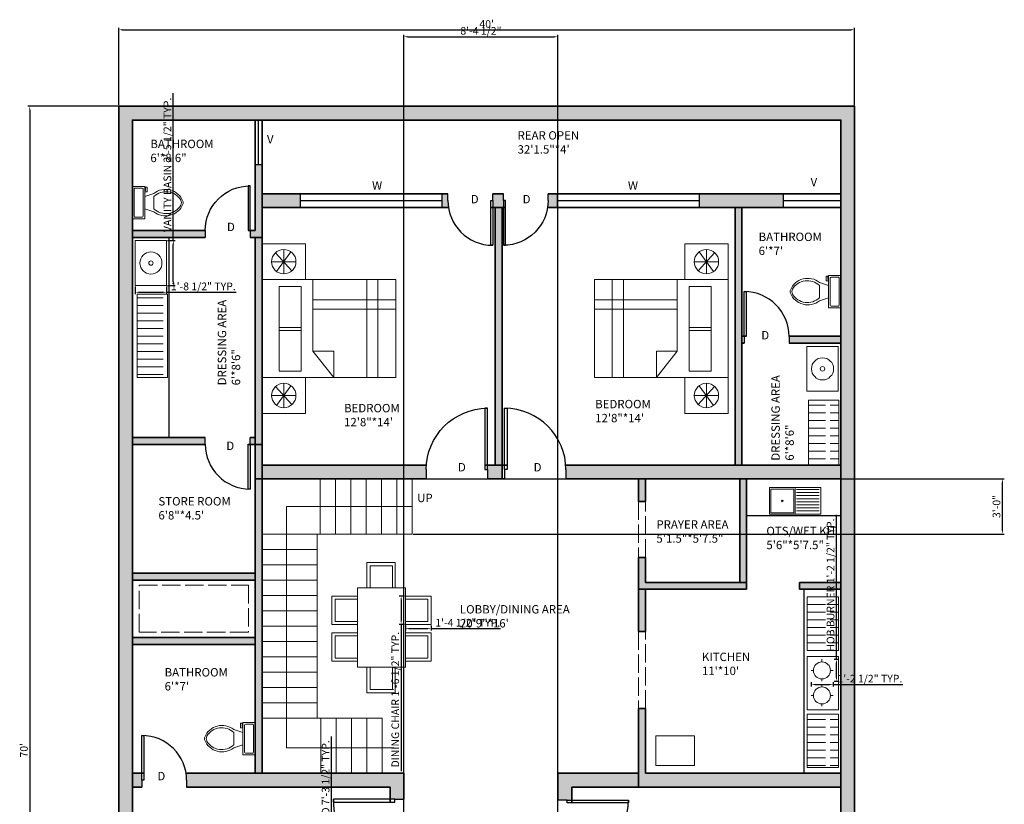
# Model space of a CAD drawing. Units: inches. Extents: x 1658 to 2301, y 1028 to 1972.
# Tile 2 of 2: x 1658 to 2301, y 1460 to 1972. Entities that reach past the tile are written whole.
import ezdxf

# ---------------------------------------------------------------- set-up
doc = ezdxf.new("R2010")
doc.units = ezdxf.units.IN
doc.linetypes.add('ACAD_ISO02W100', pattern=[15, 12, -3])
for name, color, linetype, lineweight in [('A-ANNO-DIMS', 31, 'Continuous', 18), ('A-AREA-IDEN', 31, 'Continuous', 18), ('A-EQPM', 181, 'Continuous', 18), ('A-FLOR-CASE', 181, 'Continuous', 25), ('A-FLOR-FIXT', 181, 'Continuous', 18), ('A-FLOR-FIXT-PATT', 181, 'Continuous', 13), ('A-FLOR-STRS', 104, 'Continuous', 18), ('A-WALL-OVHD', 140, 'ACAD_ISO02W100', 18), ('A-WALL-PATT', 140, 'Continuous', 13), ('DOOR', 54, 'Continuous', 25), ('FUR', 181, 'Continuous', 18), ('L-SITE-WALL', 140, 'Continuous', 35), ('TEXT', 31, 'Continuous', 18), ('WALL', 140, 'Continuous', 35), ('WIND', 211, 'Continuous', 25)]:
    doc.layers.add(name, color=color, linetype=linetype, lineweight=lineweight)
doc.styles.get("Standard").update_dxf_attribs({"font": 'arial.ttf'})
doc.dimstyles.new('ISO-25', dxfattribs={"dimtxt": 5, "dimasz": 2.5, "dimexe": 1.25, "dimexo": 0.625, "dimtad": 1, "dimdec": 0, "dimlunit": 4, "dimtxsty": 'Standard', "dimcen": 2.5, "dimadec": 0, "dimazin": 0, "dimtfac": 1, "dimtdec": 0, "dimtmove": 0, "dimatfit": 3, "dimfxl": 1, "dimarcsym": 0})

# ---------------------------------------------------------------- blocks, each defined once
blk = doc.blocks.new('*U2')
for p, q in [((0, 0), (0, -6)), ((40, 0), (40, -6))]:
    blk.add_line(p, q)
blk.add_lwpolyline([(0, 0), (0, 40), (1.75, 40), (1.75, 0)], close=True)
blk.add_arc((0, 0), 40, 0, 90)
blk = doc.blocks.new('*U4')
for p, q in [((9.5, -6), (9.5, -2)), ((-10, -8.5), (-8, -8.5)), ((-10, -9.5), (-10, -8.5)), ((-7, -9.5), (-10, -9.5)), ((-8, -8.5), (-8, -8)), ((-7, -8), (-7, -9.5)), ((-4, -8), (-6, -14)), ((4, -8), (6, -14)), ((4, -14), (-4, -14))]:
    blk.add_line(p, q)
blk.add_lwpolyline([(10.5, -8), (10.5, 0), (-10.5, 0), (-10.5, -8)], close=True)
for points in [[(-9.5, -2), (-9.5, -6)], [(8.5, -1), (-8.5, -1)], [(-8.5, -7), (8.5, -7)]]:
    blk.add_lwpolyline(points)
for centre, radius, start, end in [((-8.62, -1.88), 0.884, 81.8699, 188.1301), ((-8.62, -6.12), 0.884, 171.8699, 278.1301), ((8.62, -1.88), 0.884, 351.8699, 98.1301), ((8.62, -6.12), 0.884, 261.8699, 8.1301), ((3.52, -21.58), 12.17, 141.46911, 247.97143), ((4.2, -21.82), 11.33, 136.36773, 238.94682), ((-3.52, -21.58), 12.17, 292.02843, 38.53071), ((-4.2, -21.82), 11.33, 301.05301, 43.63209), ((0, -27.88), 4, 245.73182, 294.26817), ((0, -29), 4, 254.86053, 285.13947)]:
    blk.add_arc(centre, radius, start, end)
blk = doc.blocks.new('*D9')
at = {"layer": 'A-ANNO-DIMS', "color": 0, "lineweight": -2, "transparency": 16777216}
for p, q in [((1722.99, 1915.66), (1722.99, 1966.18)), ((2202.99, 1915.66), (2202.99, 1966.18)), ((1725.49, 1964.93), (2200.49, 1964.93))]:
    blk.add_line(p, q, dxfattribs=at)
at = {"layer": 'A-ANNO-DIMS', "color": 0, "lineweight": 100, "transparency": 16777216}
for points in [[(1725.49, 1965.34), (1725.49, 1964.51), (1722.99, 1964.93)], [(2200.49, 1965.34), (2200.49, 1964.51), (2202.99, 1964.93)]]:
    blk.add_solid(points, dxfattribs=at)
at = {"layer": 'Defpoints', "color": 0, "lineweight": 100, "transparency": 16777216}
for p in [(2202.99, 1964.93), (1722.99, 1915.04), (2202.99, 1915.04)]:
    blk.add_point(p, dxfattribs=at)
at = {"layer": 'A-ANNO-DIMS', "color": 0, "transparency": 16777216, "insert": (1962.99, 1968.1), "char_height": 5, "attachment_point": 5}
blk.add_mtext("40'", dxfattribs=at)
blk = doc.blocks.new('*D10')
at = {"layer": 'A-ANNO-DIMS', "color": 0, "lineweight": -2, "transparency": 16777216}
for p, q in [((1722.37, 1915.04), (1663.75, 1915.04)), ((1665, 1912.54), (1665, 1077.54)), ((1722.37, 1075.04), (1663.75, 1075.04))]:
    blk.add_line(p, q, dxfattribs=at)
at = {"layer": 'A-ANNO-DIMS', "color": 0, "lineweight": 100, "transparency": 16777216}
for points in [[(1664.59, 1912.54), (1665.42, 1912.54), (1665, 1915.04)], [(1664.59, 1077.54), (1665.42, 1077.54), (1665, 1075.04)]]:
    blk.add_solid(points, dxfattribs=at)
at = {"layer": 'Defpoints', "color": 0, "lineweight": 100, "transparency": 16777216}
for p in [(1722.99, 1915.04), (1665, 1075.04), (1722.99, 1075.04)]:
    blk.add_point(p, dxfattribs=at)
at = {"layer": 'A-ANNO-DIMS', "color": 0, "transparency": 16777216, "insert": (1661.82, 1495.04), "char_height": 5, "attachment_point": 5, "rotation": 90}
blk.add_mtext("70'", dxfattribs=at)
blk = doc.blocks.new('BED-DOUBLE')
for p, q in [((33.2, 63.87), (33.2, 17.24)), ((68.25, 63.87), (68.25, 0)), ((75.56, 63.87), (75.56, 0)), ((33.2, 50.75), (87.28, 50.75)), ((33.2, 44.52), (87.28, 44.52)), ((33.2, 17.24), (46.75, 17.24)), ((46.75, 0), (33.2, 17.24)), ((46.75, 17.24), (46.75, 0))]:
    blk.add_line(p, q)
for points in [[(0, 0), (87.28, 0), (87.28, 63.87), (0, 63.87)], [(11.05, 30.77), (25.46, 30.77), (25.46, 59.34), (11.05, 59.34)], [(11.05, 4.13), (25.46, 4.13), (25.46, 32.7), (11.05, 32.7)]]:
    blk.add_lwpolyline(points, close=True)
blk = doc.blocks.new('NIGHTSTAND-LAMP')
for p, q in [((14.17, 3.75), (14.17, 19.65)), ((19.52, 5.82), (8.81, 17.58)), ((9.46, 5.29), (18.87, 18.1)), ((6.22, 11.7), (22.11, 11.7))]:
    blk.add_line(p, q)
blk.add_lwpolyline([(0, 0), (28.33, 0), (28.33, 23.39), (0, 23.39)], close=True)
blk.add_circle((14.17, 11.7), 7.95)
blk = doc.blocks.new('DINING-CHAIR')
for p, q in [((0, 0), (0, 16.69)), ((0, 16.69), (18.47, 16.69)), ((18.47, 16.69), (18.47, 0))]:
    blk.add_line(p, q)
blk.add_lwpolyline([(2.01, 0), (16.57, 0), (16.57, 14.56), (2.01, 14.56)], close=True)
blk = doc.blocks.new('VANITY-BASIN')
blk.add_lwpolyline([(0, 29.33), (20.39, 29.33), (20.39, 0), (0, 0)], close=True)
for radius in [7.21, 1.43]:
    blk.add_circle((10.2, 14.66), radius)
blk = doc.blocks.new('HOB-BURNER')
for p, q in [((7.04, 12.61), (7.04, 14.41)), ((1.5, 7.07), (0, 7.07)), ((12.57, 7.07), (14.33, 7.07)), ((7.04, 1.54), (7.04, 0))]:
    blk.add_line(p, q)
blk.add_circle((7.04, 7.07), 5.54)
blk = doc.blocks.new('*D17')
at = {"layer": 'A-ANNO-DIMS', "color": 0, "lineweight": -2, "transparency": 16777216}
for p, q in [((1861.79, 1411.32), (1861.79, 1503.92)), ((1849.32, 1411.32), (1863.04, 1411.32)), ((1861.79, 1326.54), (1861.79, 1408.82)), ((1849.32, 1324.04), (1863.04, 1324.04))]:
    blk.add_line(p, q, dxfattribs=at)
at = {"layer": 'A-ANNO-DIMS', "color": 0, "lineweight": 100, "transparency": 16777216}
for points in [[(1861.37, 1408.82), (1862.2, 1408.82), (1861.79, 1411.32)], [(1861.37, 1326.54), (1862.2, 1326.54), (1861.79, 1324.04)]]:
    blk.add_solid(points, dxfattribs=at)
at = {"layer": 'Defpoints', "color": 0, "lineweight": 100, "transparency": 16777216}
for p in [(1848.69, 1411.32), (1861.79, 1411.32), (1848.69, 1324.04)]:
    blk.add_point(p, dxfattribs=at)
at = {"layer": 'A-ANNO-DIMS', "color": 0, "transparency": 16777216, "insert": (1858.57, 1458.87), "char_height": 5, "attachment_point": 5, "rotation": 90}
blk.add_mtext('DOUBLE BED 7\'-3 1/2" TYP.', dxfattribs=at)
blk = doc.blocks.new('*D21')
at = {"layer": 'A-ANNO-DIMS', "color": 0, "lineweight": -2, "transparency": 16777216}
for p, q in [((1909.36, 1595.59), (1905.97, 1595.59)), ((1907.22, 1593.09), (1907.22, 1579.62)), ((1909.36, 1577.12), (1905.97, 1577.12)), ((1907.22, 1577.12), (1907.22, 1481.43))]:
    blk.add_line(p, q, dxfattribs=at)
at = {"layer": 'A-ANNO-DIMS', "color": 0, "lineweight": 100, "transparency": 16777216}
for points in [[(1906.8, 1593.09), (1907.63, 1593.09), (1907.22, 1595.59)], [(1906.8, 1579.62), (1907.63, 1579.62), (1907.22, 1577.12)]]:
    blk.add_solid(points, dxfattribs=at)
at = {"layer": 'Defpoints', "color": 0, "lineweight": 100, "transparency": 16777216}
for p in [(1909.99, 1595.59), (1907.22, 1577.12), (1909.99, 1577.12)]:
    blk.add_point(p, dxfattribs=at)
at = {"layer": 'A-ANNO-DIMS', "color": 0, "transparency": 16777216, "insert": (1904.01, 1528.03), "char_height": 5, "attachment_point": 5, "rotation": 90}
blk.add_mtext('DINING CHAIR 1\'-6 1/2" TYP.', dxfattribs=at)
blk = doc.blocks.new('*D22')
at = {"layer": 'A-ANNO-DIMS', "color": 0, "lineweight": -2, "transparency": 16777216}
for p, q in [((1909.99, 1576.5), (1909.99, 1573.1)), ((1912.49, 1574.35), (1924.18, 1574.35)), ((1926.68, 1576.5), (1926.68, 1573.1)), ((1926.68, 1574.35), (1972.08, 1574.35))]:
    blk.add_line(p, q, dxfattribs=at)
at = {"layer": 'A-ANNO-DIMS', "color": 0, "lineweight": 100, "transparency": 16777216}
for points in [[(1912.49, 1574.77), (1912.49, 1573.93), (1909.99, 1574.35)], [(1924.18, 1574.77), (1924.18, 1573.93), (1926.68, 1574.35)]]:
    blk.add_solid(points, dxfattribs=at)
at = {"layer": 'Defpoints', "color": 0, "lineweight": 100, "transparency": 16777216}
for p in [(1909.99, 1577.12), (1926.68, 1577.12), (1926.68, 1574.35)]:
    blk.add_point(p, dxfattribs=at)
at = {"layer": 'A-ANNO-DIMS', "color": 0, "transparency": 16777216, "insert": (1950.63, 1577.56), "char_height": 5, "attachment_point": 5}
blk.add_mtext('1\'-4 1/2" TYP.', dxfattribs=at)
blk = doc.blocks.new('*D25')
at = {"layer": 'A-ANNO-DIMS', "color": 0, "lineweight": -2, "transparency": 16777216}
for p, q in [((1758.61, 1827.46), (1758.61, 1923.67)), ((1754.84, 1827.46), (1759.86, 1827.46)), ((1758.61, 1800.63), (1758.61, 1824.96)), ((1754.84, 1798.13), (1759.86, 1798.13))]:
    blk.add_line(p, q, dxfattribs=at)
at = {"layer": 'A-ANNO-DIMS', "color": 0, "lineweight": 100, "transparency": 16777216}
for points in [[(1758.2, 1824.96), (1759.03, 1824.96), (1758.61, 1827.46)], [(1758.2, 1800.63), (1759.03, 1800.63), (1758.61, 1798.13)]]:
    blk.add_solid(points, dxfattribs=at)
at = {"layer": 'Defpoints', "color": 0, "lineweight": 100, "transparency": 16777216}
for p in [(1754.21, 1827.46), (1758.61, 1827.46), (1754.21, 1798.13)]:
    blk.add_point(p, dxfattribs=at)
at = {"layer": 'A-ANNO-DIMS', "color": 0, "transparency": 16777216, "insert": (1755.4, 1876.82), "char_height": 5, "attachment_point": 5, "rotation": 90}
blk.add_mtext('VANITY BASIN 2\'-5 1/2" TYP.', dxfattribs=at)
blk = doc.blocks.new('*D26')
at = {"layer": 'A-ANNO-DIMS', "color": 0, "lineweight": -2, "transparency": 16777216}
for p, q in [((1733.82, 1797.51), (1733.82, 1792.48)), ((1736.32, 1793.73), (1751.71, 1793.73)), ((1754.21, 1797.51), (1754.21, 1792.48)), ((1754.21, 1793.73), (1799.62, 1793.73))]:
    blk.add_line(p, q, dxfattribs=at)
at = {"layer": 'A-ANNO-DIMS', "color": 0, "lineweight": 100, "transparency": 16777216}
for points in [[(1736.32, 1794.15), (1736.32, 1793.32), (1733.82, 1793.73)], [(1751.71, 1794.15), (1751.71, 1793.32), (1754.21, 1793.73)]]:
    blk.add_solid(points, dxfattribs=at)
at = {"layer": 'Defpoints', "color": 0, "lineweight": 100, "transparency": 16777216}
for p in [(1733.82, 1798.13), (1754.21, 1798.13), (1754.21, 1793.73)]:
    blk.add_point(p, dxfattribs=at)
at = {"layer": 'A-ANNO-DIMS', "color": 0, "transparency": 16777216, "insert": (1778.17, 1796.94), "char_height": 5, "attachment_point": 5}
blk.add_mtext('1\'-8 1/2" TYP.', dxfattribs=at)
blk = doc.blocks.new('*D27')
at = {"layer": 'A-ANNO-DIMS', "color": 0, "lineweight": -2, "transparency": 16777216}
for p, q in [((2191.13, 1554.45), (2191.13, 1648.57)), ((2189.59, 1554.45), (2192.38, 1554.45)), ((2191.13, 1542.54), (2191.13, 1551.95)), ((2189.59, 1540.04), (2192.38, 1540.04))]:
    blk.add_line(p, q, dxfattribs=at)
at = {"layer": 'A-ANNO-DIMS', "color": 0, "lineweight": 100, "transparency": 16777216}
for points in [[(2190.71, 1551.95), (2191.54, 1551.95), (2191.13, 1554.45)], [(2190.71, 1542.54), (2191.54, 1542.54), (2191.13, 1540.04)]]:
    blk.add_solid(points, dxfattribs=at)
at = {"layer": 'Defpoints', "color": 0, "lineweight": 100, "transparency": 16777216}
for p in [(2188.96, 1554.45), (2191.13, 1554.45), (2188.96, 1540.04)]:
    blk.add_point(p, dxfattribs=at)
at = {"layer": 'A-ANNO-DIMS', "color": 0, "transparency": 16777216, "insert": (2187.91, 1602.76), "char_height": 5, "attachment_point": 5, "rotation": 90}
blk.add_mtext('HOB BURNER 1\'-2 1/2" TYP.', dxfattribs=at)
blk = doc.blocks.new('*D28')
at = {"layer": 'A-ANNO-DIMS', "color": 0, "lineweight": -2, "transparency": 16777216}
for p, q in [((2174.64, 1539.41), (2174.64, 1536.63)), ((2177.14, 1537.88), (2186.46, 1537.88)), ((2188.96, 1539.41), (2188.96, 1536.63)), ((2188.96, 1537.88), (2234.37, 1537.88))]:
    blk.add_line(p, q, dxfattribs=at)
at = {"layer": 'A-ANNO-DIMS', "color": 0, "lineweight": 100, "transparency": 16777216}
for points in [[(2177.14, 1538.29), (2177.14, 1537.46), (2174.64, 1537.88)], [(2186.46, 1538.29), (2186.46, 1537.46), (2188.96, 1537.88)]]:
    blk.add_solid(points, dxfattribs=at)
at = {"layer": 'Defpoints', "color": 0, "lineweight": 100, "transparency": 16777216}
for p in [(2174.64, 1540.04), (2188.96, 1540.04), (2188.96, 1537.88)]:
    blk.add_point(p, dxfattribs=at)
at = {"layer": 'A-ANNO-DIMS', "color": 0, "transparency": 16777216, "insert": (2212.92, 1541.09), "char_height": 5, "attachment_point": 5}
blk.add_mtext('1\'-2 1/2" TYP.', dxfattribs=at)
blk = doc.blocks.new('*D31')
at = {"layer": 'A-ANNO-DIMS', "color": 0, "lineweight": -2, "transparency": 16777216}
for p, q in [((1908.99, 1357.76), (1908.99, 1961.64)), ((1911.49, 1960.39), (2006.99, 1960.39)), ((2009.49, 1357.76), (2009.49, 1961.64))]:
    blk.add_line(p, q, dxfattribs=at)
at = {"layer": 'A-ANNO-DIMS', "color": 0, "lineweight": 100, "transparency": 16777216}
for points in [[(1911.49, 1960.8), (1911.49, 1959.97), (1908.99, 1960.39)], [(2006.99, 1960.8), (2006.99, 1959.97), (2009.49, 1960.39)]]:
    blk.add_solid(points, dxfattribs=at)
at = {"layer": 'Defpoints', "color": 0, "lineweight": 100, "transparency": 16777216}
for p in [(2009.49, 1960.39), (1908.99, 1357.13), (2009.49, 1357.13)]:
    blk.add_point(p, dxfattribs=at)
at = {"layer": 'A-ANNO-DIMS', "color": 0, "transparency": 16777216, "insert": (1959.24, 1963.6), "char_height": 5, "attachment_point": 5}
blk.add_mtext('8\'-4 1/2"', dxfattribs=at)
blk = doc.blocks.new('*D33')
at = {"layer": 'A-ANNO-DIMS', "color": 0, "lineweight": -2, "transparency": 16777216}
for p, q in [((1915.04, 1672.04), (2300.59, 1672.04)), ((2299.34, 1638.54), (2299.34, 1669.54)), ((1915.04, 1636.04), (2300.59, 1636.04))]:
    blk.add_line(p, q, dxfattribs=at)
at = {"layer": 'A-ANNO-DIMS', "color": 0, "lineweight": 100, "transparency": 16777216}
for points in [[(2298.92, 1669.54), (2299.76, 1669.54), (2299.34, 1672.04)], [(2298.92, 1638.54), (2299.76, 1638.54), (2299.34, 1636.04)]]:
    blk.add_solid(points, dxfattribs=at)
at = {"layer": 'Defpoints', "color": 0, "lineweight": 100, "transparency": 16777216}
for p in [(1914.41, 1672.04), (2299.34, 1672.04), (1914.41, 1636.04)]:
    blk.add_point(p, dxfattribs=at)
at = {"layer": 'A-ANNO-DIMS', "color": 0, "transparency": 16777216, "insert": (2296.16, 1654.04), "char_height": 5, "attachment_point": 5, "rotation": 90}
blk.add_mtext('3\'-0"', dxfattribs=at)

msp = doc.modelspace()

# ---------------------------------------------------------------- hatches: boundary and pattern name
at = {"layer": 'A-FLOR-FIXT-PATT'}
h = msp.add_hatch(dxfattribs=at)
h.set_pattern_fill('ACAD_ISO08W100', color=256)
h.paths.add_polyline_path([(1754.74, 1792.4), (1734.94, 1792.4), (1734.94, 1738.22), (1754.74, 1738.22)])
h = msp.add_hatch(dxfattribs=at)
h.set_pattern_fill('ACAD_ISO08W100', color=256)
h.paths.add_polyline_path([(2192.74, 1723.4), (2172.94, 1723.4), (2172.94, 1681.04), (2192.74, 1681.04)])
h = msp.add_hatch(dxfattribs=at)
h.set_pattern_fill('ACAD_ISO08W100', color=256)
h.paths.add_polyline_path([(2192.44, 1595), (2171.93, 1595), (2171.93, 1560.13), (2192.44, 1560.13)])
h.paths.add_polyline_path([(2192.44, 1518.57), (2171.93, 1518.57), (2171.93, 1483.7), (2192.44, 1483.7)])
at = {"layer": 'A-WALL-PATT'}
h = msp.add_hatch(color=256, dxfattribs=at)
h.dxf.hatch_style = 1
h.paths.add_polyline_path([(1731.99, 1315.04), (1731.99, 1906.04), (2193.99, 1906.04), (2193.99, 1084.04), (1870.11, 1084.04), (1870.11, 1075.04), (2202.99, 1075.04), (2202.99, 1915.04), (1722.99, 1915.04), (1722.99, 1075.04), (1731.99, 1075.04), (1731.99, 1084.04)])
h = msp.add_hatch(color=256, dxfattribs=at)
h.dxf.hatch_style = 1
h.paths.add_polyline_path([(1779.42, 1699.04), (1731.99, 1699.04), (1731.99, 1697.54), (1731.99, 1694.54), (1779.42, 1694.54)])
h.paths.add_polyline_path([(1816.49, 1672.04), (1811.99, 1672.04), (1811.99, 1640.54), (1811.99, 1480.04), (1816.49, 1480.04)])
h.paths.add_polyline_path([(1811.99, 1610.54), (1731.99, 1610.54), (1731.99, 1606.04), (1811.99, 1606.04)])
h.paths.add_polyline_path([(1811.99, 1568.54), (1731.99, 1568.54), (1731.99, 1564.04), (1811.99, 1564.04)])
h.paths.add_polyline_path([(1738.02, 1480.04), (1731.99, 1480.04), (1731.99, 1471.04), (1738.02, 1471.04), (1738.02, 1475.43)])
h.paths.add_polyline_path([(1908.99, 1480.04), (1766.9, 1480.04, -0.039614), (1767.27, 1475.43), (1767.27, 1471.04), (1899.99, 1471.04), (1899.99, 1463.03), (1902.99, 1463.03), (1908.99, 1463.03)])
h.paths.add_polyline_path([(1908.99, 1423.03), (1902.99, 1423.03, -0.01877), (1899.99, 1423.14), (1899.99, 1324.04), (1863.03, 1324.04), (1863.03, 1315.04), (1908.99, 1315.04)])
h.paths.add_polyline_path([(1770.21, 1324.04), (1761.43, 1324.04), (1731.99, 1324.04), (1731.99, 1315.04), (1770.21, 1315.04)])
h.paths.add_polyline_path([(2009.49, 1357.13), (1988.35, 1357.13), (1988.35, 1352.34), (1988.35, 1348.13), (2009.49, 1348.13)])
h.paths.add_polyline_path([(1932.24, 1352.34), (1932.24, 1357.13), (1908.99, 1357.13), (1908.99, 1348.13), (1932.24, 1348.13)])
h.paths.add_polyline_path([(2018.49, 1422.69, -0.01877), (2015.49, 1422.57), (2009.49, 1422.57), (2009.49, 1328.83), (2015.49, 1328.83, -0.01877), (2018.49, 1328.71)])
h.paths.add_polyline_path([(2054.42, 1279.04), (2018.49, 1279.04), (2009.49, 1279.04), (2009.49, 1270.04), (2054.42, 1270.04)])
h.paths.add_polyline_path([(2018.49, 1288.83), (2015.49, 1288.83), (2009.49, 1288.83), (2009.49, 1279.04), (2018.49, 1279.04)])
h.paths.add_polyline_path([(2193.99, 1279.04), (2147.24, 1279.04), (2147.24, 1270.04), (2193.99, 1270.04)])
h.paths.add_polyline_path([(2061.99, 1480.04), (2009.49, 1480.04), (2009.49, 1462.57), (2015.49, 1462.57), (2018.49, 1462.57), (2018.49, 1471.04), (2061.99, 1471.04)])
h.paths.add_polyline_path([(2193.99, 1480.04), (2169.99, 1480.04), (2066.49, 1480.04), (2066.49, 1522.24), (2061.99, 1522.24), (2061.99, 1471.04), (2193.99, 1471.04)])
h.paths.add_polyline_path([(2066.49, 1600.04), (2061.99, 1600.04), (2061.99, 1572.51), (2066.49, 1572.51)])
h.paths.add_polyline_path([(2066.49, 1672.04), (2061.99, 1672.04), (2061.99, 1657.22), (2066.49, 1657.22)])
h.paths.add_polyline_path([(2132.49, 1604.54), (2127.99, 1604.54), (2066.49, 1604.54), (2066.49, 1620.73), (2061.99, 1620.73), (2061.99, 1600.04), (2132.49, 1600.04)])
h.paths.add_polyline_path([(2132.49, 1672.04), (2127.99, 1672.04), (2127.99, 1604.54), (2132.49, 1604.54)])
h.paths.add_polyline_path([(2193.99, 1604.54), (2166.96, 1604.54), (2166.96, 1600.04), (2193.99, 1600.04)])
h.paths.add_polyline_path([(2193.99, 1681.04), (2014.55, 1681.04, -0.01877), (2014.67, 1678.04), (2014.67, 1672.04), (2193.99, 1672.04)])
h.paths.add_polyline_path([(2166.4, 1681.92), (2166.4, 1747.55), (2145.97, 1747.55), (2145.97, 1681.92)], flags=9)
h.paths.add_polyline_path([(1915.65, 1653.85), (1929.01, 1653.85), (1929.01, 1665.13), (1915.65, 1665.13)], flags=9)
h.paths.add_polyline_path([(2138.45, 1814.92), (2185.37, 1814.92), (2185.37, 1835.35), (2138.45, 1835.35)], flags=9)
h.paths.add_polyline_path([(1981.17, 1881.08), (2028.95, 1881.08), (2028.95, 1901.5), (1981.17, 1901.5)], flags=9)
h.paths.add_polyline_path([(1867.78, 1703.2), (1910.3, 1703.2), (1910.3, 1723.63), (1867.78, 1723.63)], flags=9)
h.paths.add_polyline_path([(2031.55, 1705.85), (2074.07, 1705.85), (2074.07, 1726.27), (2031.55, 1726.27)], flags=9)
h.paths.add_polyline_path([(1943.61, 1572), (2023.69, 1572), (2023.69, 1592.42), (1943.61, 1592.42)], flags=9)
h.paths.add_polyline_path([(2071.73, 1627.4), (2128.87, 1627.4), (2128.87, 1647.83), (2071.73, 1647.83)], flags=9)
h.paths.add_polyline_path([(2143.67, 1623.1), (2195.26, 1623.1), (2195.26, 1643.52), (2143.67, 1643.52)], flags=9)
h.paths.add_polyline_path([(2101.19, 1540.97), (2137.76, 1540.97), (2137.76, 1561.39), (2101.19, 1561.39)], flags=9)
h.paths.add_polyline_path([(2091.03, 1326.07), (2156.87, 1326.07), (2156.87, 1346.5), (2091.03, 1346.5)], flags=9)
h.paths.add_polyline_path([(1796.89, 1432.36), (1852.31, 1432.36), (1852.31, 1452.79), (1796.89, 1452.79)], flags=9)
h.paths.add_polyline_path([(1751.02, 1530.9), (1797.94, 1530.9), (1797.94, 1551.32), (1751.02, 1551.32)], flags=9)
h.paths.add_polyline_path([(1747.18, 1642.43), (1802.17, 1642.43), (1802.17, 1662.86), (1747.18, 1662.86)], flags=9)
h.paths.add_polyline_path([(1805.32, 1731.07), (1805.32, 1796.71), (1784.9, 1796.71), (1784.9, 1731.07)], flags=9)
h.paths.add_polyline_path([(1741.72, 1875.52), (1788.64, 1875.52), (1788.64, 1895.95), (1741.72, 1895.95)], flags=9)
h = msp.add_hatch(color=256, dxfattribs=at)
h.dxf.hatch_style = 1
h.paths.add_polyline_path([(1816.49, 1829.54), (1811.99, 1829.54), (1811.99, 1757.54), (1811.99, 1753.04), (1811.99, 1699.04), (1811.99, 1694.54), (1816.49, 1694.54)])
h.paths.add_polyline_path([(1779.42, 1834.04), (1731.99, 1834.04), (1731.99, 1829.54), (1779.42, 1829.54)])
h.paths.add_polyline_path([(1816.49, 1876.97), (1811.99, 1876.97), (1811.99, 1834.04), (1808.67, 1834.04), (1808.67, 1833.93), (1808.67, 1829.54), (1811.99, 1829.54), (1816.49, 1829.54)])
h = msp.add_hatch(color=256, dxfattribs=at)
h.dxf.hatch_style = 1
h.paths.add_polyline_path([(1841.24, 1858.04), (1816.49, 1858.04), (1816.49, 1849.04), (1841.24, 1849.04)])
h.paths.add_polyline_path([(1937.66, 1858.04), (1934.06, 1858.04), (1934.06, 1849.04), (1938.03, 1849.04, -0.039614), (1937.66, 1853.65)])
h.paths.add_polyline_path([(1973.88, 1853.65), (1973.88, 1858.04), (1966.91, 1858.04), (1966.91, 1853.65), (1966.91, 1849.04), (1973.88, 1849.04)])
h.paths.add_polyline_path([(2008.9, 1858.04), (2003.13, 1858.04), (2003.13, 1853.65, -0.039614), (2002.76, 1849.04), (2008.9, 1849.04)])
h.paths.add_polyline_path([(2156.35, 1858.04), (2101.72, 1858.04), (2101.72, 1849.04), (2156.35, 1849.04)])
h.paths.add_polyline_path([(2129.49, 1849.04), (2124.99, 1849.04), (2124.99, 1681.04), (2129.49, 1681.04)])
h.paths.add_polyline_path([(1972.99, 1849.04), (1968.49, 1849.04), (1968.49, 1681.04), (1972.99, 1681.04)])
h.paths.add_polyline_path([(1923.68, 1681.04), (1816.49, 1681.04), (1816.49, 1672.04), (1923.57, 1672.04), (1923.57, 1678.04, -0.01877)])
h.paths.add_polyline_path([(1811.99, 1699.04), (1808.67, 1699.04), (1808.67, 1694.54), (1811.99, 1694.54)])
h.paths.add_polyline_path([(1816.49, 1694.54), (1811.99, 1694.54), (1811.99, 1672.04), (1816.49, 1672.04), (1816.49, 1681.04)])
h = msp.add_hatch(color=256, dxfattribs=at)
h.dxf.hatch_style = 1
h.paths.add_polyline_path([(2193.99, 1765.04), (2160.21, 1765.04), (2160.21, 1760.54), (2193.99, 1760.54)])
h = msp.add_hatch(color=256, dxfattribs=at)
h.dxf.hatch_style = 1
h.paths.add_polyline_path([(1972.99, 1681.04), (1968.49, 1681.04), (1963.57, 1681.04), (1963.57, 1678.04), (1963.57, 1672.04), (1972.99, 1672.04)])

# ---------------------------------------------------------------- linework, layer by layer
at = {"layer": 'A-EQPM'}
for points in [[(2171.93, 1521.34), (2192.44, 1521.34), (2192.44, 1556.21), (2171.93, 1556.21)], [(2073.35, 1485.09), (2098.5, 1485.09), (2098.5, 1504.42), (2073.35, 1504.42)]]:
    msp.add_lwpolyline(points, close=True, dxfattribs=at)
at = {"layer": 'A-FLOR-CASE'}
for p, q in [((1755.99, 1699.04), (1755.99, 1829.54)), ((2193.99, 1630.04), (2193.99, 1760.54)), ((1731.99, 1699.04), (1755.99, 1699.04)), ((2132.49, 1672.04), (2132.49, 1648.04)), ((2132.49, 1648.04), (2193.99, 1648.04)), ((2169.99, 1578.87), (2169.99, 1600.04)), ((2169.99, 1480.04), (2169.99, 1578.87)), ((2193.99, 1480.04), (2169.99, 1480.04))]:
    msp.add_line(p, q, dxfattribs=at)
at = {"layer": 'A-FLOR-FIXT'}
for p, q in [((2164.17, 1649.12), (2164.17, 1666.35)), ((2164.97, 1665.11), (2179.85, 1665.11)), ((2164.97, 1663.11), (2179.85, 1663.11)), ((2164.97, 1661.11), (2179.85, 1661.11)), ((2164.97, 1659.11), (2179.85, 1659.11)), ((2164.97, 1657.11), (2179.85, 1657.11)), ((2164.97, 1655.11), (2179.85, 1655.11)), ((2164.97, 1653.11), (2179.85, 1653.11)), ((2164.97, 1651.11), (2179.85, 1651.11))]:
    msp.add_line(p, q, dxfattribs=at)
for points in [[(1734.94, 1792.4), (1754.74, 1792.4), (1754.74, 1738.22), (1734.94, 1738.22)], [(2147.46, 1649.12), (2180.88, 1649.12), (2180.88, 1666.35), (2147.46, 1666.35)], [(2148.23, 1665.35), (2163.39, 1665.35), (2163.39, 1649.91), (2148.23, 1649.91)], [(2171.93, 1560.13), (2192.44, 1560.13), (2192.44, 1595), (2171.93, 1595)], [(2171.93, 1483.7), (2192.44, 1483.7), (2192.44, 1518.57), (2171.93, 1518.57)]]:
    msp.add_lwpolyline(points, close=True, dxfattribs=at)
msp.add_lwpolyline([(2172.94, 1681.04), (2172.94, 1723.4), (2192.74, 1723.4), (2192.74, 1681.04)], dxfattribs=at)
msp.add_circle((2155.81, 1657.63), 0.502, dxfattribs=at)
at = {"layer": 'A-FLOR-STRS'}
for p, q in [((1854.41, 1672.04), (1854.41, 1636.04)), ((1864.41, 1672.04), (1864.41, 1636.04)), ((1874.41, 1672.04), (1874.41, 1636.04)), ((1884.41, 1672.04), (1884.41, 1636.04)), ((1894.41, 1672.04), (1894.41, 1636.04)), ((1904.41, 1672.04), (1904.41, 1636.04)), ((1914.41, 1672.04), (1914.41, 1636.04)), ((1914.41, 1654.04), (1832.45, 1654.04)), ((1832.45, 1654.04), (1832.45, 1496.68)), ((1852.49, 1636.04), (1816.49, 1636.04)), ((1914.41, 1636.04), (1852.49, 1636.04)), ((1852.49, 1516.04), (1852.49, 1636.04)), ((1852.49, 1626.04), (1816.49, 1626.04)), ((1852.49, 1616.04), (1816.49, 1616.04)), ((1852.49, 1606.04), (1816.49, 1606.04)), ((1852.49, 1596.04), (1816.49, 1596.04)), ((1852.49, 1586.04), (1816.49, 1586.04)), ((1852.49, 1576.04), (1816.49, 1576.04)), ((1852.49, 1566.04), (1816.49, 1566.04)), ((1852.49, 1556.04), (1816.49, 1556.04)), ((1852.49, 1546.04), (1816.49, 1546.04)), ((1852.49, 1536.04), (1816.49, 1536.04)), ((1852.49, 1526.04), (1816.49, 1526.04)), ((1852.49, 1516.04), (1816.49, 1516.04)), ((1894.81, 1516.04), (1852.49, 1516.04)), ((1854.81, 1480.04), (1854.81, 1516.04)), ((1864.81, 1480.04), (1864.81, 1516.04)), ((1874.81, 1480.04), (1874.81, 1516.04)), ((1884.81, 1480.04), (1884.81, 1516.04)), ((1894.81, 1480.04), (1894.81, 1516.04)), ((1832.45, 1496.68), (1902.7, 1496.68))]:
    msp.add_line(p, q, dxfattribs=at)
at = {"layer": 'A-WALL-OVHD'}
for points in [[(2061.99, 1620.73), (2066.49, 1620.73), (2066.49, 1657.22), (2061.99, 1657.22)], [(1736.35, 1602.68), (1807.58, 1602.68), (1807.58, 1571.96), (1736.35, 1571.96)], [(2061.99, 1522.24), (2066.49, 1522.24), (2066.49, 1572.51), (2061.99, 1572.51)]]:
    msp.add_lwpolyline(points, close=True, dxfattribs=at)
at = {"layer": 'FUR'}
msp.add_lwpolyline([(1878.72, 1600.86), (1909.99, 1600.86), (1909.99, 1549.19), (1878.72, 1549.19)], close=True, dxfattribs=at)
at = {"layer": 'L-SITE-WALL'}
for p, q in [((1722.99, 1915.04), (2202.99, 1915.04)), ((1722.99, 1075.04), (1722.99, 1915.04)), ((2202.99, 1915.04), (2202.99, 1075.04))]:
    msp.add_line(p, q, dxfattribs=at)
for points in [[(1731.99, 1075.04), (1722.99, 1075.04), (1722.99, 1915.04), (2202.99, 1915.04), (2202.99, 1075.04), (1870.11, 1075.04)], [(1731.99, 1084.04), (1731.99, 1906.04), (2193.99, 1906.04), (2193.99, 1084.04), (1870.11, 1084.04)]]:
    msp.add_lwpolyline(points, dxfattribs=at)
at = {"layer": 'WALL'}
for p, q in [((1731.99, 1906.04), (1803.99, 1906.04)), ((1731.99, 1906.04), (1811.99, 1906.04)), ((1811.99, 1906.04), (1811.99, 1834.04)), ((1816.49, 1906.04), (1816.49, 1829.54)), ((1816.49, 1906.04), (1816.49, 1858.04)), ((1816.49, 1858.04), (1937.66, 1858.04)), ((1966.91, 1858.04), (1973.88, 1858.04)), ((2003.13, 1858.04), (2193.99, 1858.04)), ((1816.49, 1849.04), (1938.03, 1849.04)), ((1816.49, 1849.04), (1816.49, 1681.04)), ((1965.63, 1849.04), (1975.16, 1849.04)), ((1968.49, 1681.04), (1968.49, 1849.04)), ((1972.99, 1672.04), (1972.99, 1849.04)), ((2002.76, 1849.04), (2193.99, 1849.04)), ((2124.99, 1681.04), (2124.99, 1849.04)), ((2129.49, 1681.04), (2129.49, 1849.04)), ((2129.49, 1849.04), (2129.49, 1765.04)), ((1739.99, 1834.04), (1731.99, 1834.04)), ((1779.42, 1834.04), (1731.99, 1834.04)), ((1811.99, 1834.04), (1807.39, 1834.04)), ((1731.99, 1829.54), (1779.42, 1829.54)), ((1731.99, 1829.54), (1779.42, 1829.54)), ((1779.42, 1829.54), (1731.99, 1829.54)), ((1816.49, 1829.54), (1808.67, 1829.54)), ((1808.67, 1829.54), (1811.99, 1829.54)), ((1808.67, 1829.54), (1811.99, 1829.54)), ((1811.99, 1829.54), (1811.99, 1757.54)), ((1816.49, 1829.54), (1816.49, 1753.04)), ((1731.99, 1799.54), (1731.99, 1697.54)), ((2129.49, 1765.04), (2132.24, 1765.04)), ((2129.49, 1760.54), (2130.96, 1760.54)), ((2160.21, 1765.04), (2193.99, 1765.04)), ((2160.21, 1760.54), (2193.99, 1760.54)), ((1811.99, 1757.54), (1811.99, 1753.04)), ((1731.99, 1753.04), (1731.99, 1699.04)), ((1811.99, 1699.04), (1811.99, 1753.04)), ((1816.49, 1694.54), (1816.49, 1753.04)), ((1731.99, 1699.04), (1779.42, 1699.04)), ((1808.67, 1699.04), (1811.99, 1699.04)), ((1811.99, 1699.04), (1811.99, 1672.04)), ((1731.99, 1694.54), (1779.42, 1694.54)), ((1731.99, 1694.54), (1779.42, 1694.54)), ((1731.99, 1694.54), (1731.99, 1610.54)), ((1807.39, 1694.54), (1811.99, 1694.54)), ((1807.39, 1694.54), (1816.49, 1694.54)), ((1811.99, 1694.54), (1811.99, 1640.54)), ((1816.49, 1681.04), (1923.68, 1681.04)), ((1816.49, 1681.04), (1816.49, 1480.04)), ((1961.82, 1681.04), (1968.49, 1681.04)), ((1968.49, 1681.04), (1976.42, 1681.04)), ((1972.99, 1681.04), (1976.42, 1681.04)), ((2014.55, 1681.04), (2124.99, 1681.04)), ((2014.55, 1681.04), (2193.99, 1681.04)), ((1811.99, 1672.04), (1923.57, 1672.04)), ((1963.57, 1672.04), (1972.99, 1672.04)), ((1972.99, 1672.04), (1974.67, 1672.04)), ((2014.67, 1672.04), (2193.99, 1672.04)), ((2061.99, 1672.04), (2061.99, 1657.22)), ((2066.49, 1672.04), (2066.49, 1657.22)), ((2193.99, 1672.04), (2127.99, 1672.04)), ((2127.99, 1604.54), (2127.99, 1672.04)), ((2132.49, 1600.04), (2132.49, 1672.04)), ((1811.99, 1640.54), (1811.99, 1480.04)), ((2061.99, 1620.73), (2061.99, 1600.04)), ((2066.49, 1620.73), (2066.49, 1604.54)), ((1731.99, 1610.54), (1811.99, 1610.54)), ((1731.99, 1606.04), (1811.99, 1606.04)), ((2061.99, 1600.04), (2132.49, 1600.04)), ((2061.99, 1600.04), (2061.99, 1572.51)), ((2066.49, 1604.54), (2127.99, 1604.54)), ((2066.49, 1600.04), (2066.49, 1572.51)), ((2127.99, 1604.54), (2132.49, 1604.54)), ((2166.96, 1604.54), (2193.99, 1604.54)), ((2166.96, 1604.54), (2166.96, 1600.04)), ((2166.96, 1600.04), (2193.99, 1600.04)), ((1731.99, 1568.54), (1811.99, 1568.54)), ((1731.99, 1480.04), (1731.99, 1564.04)), ((1731.99, 1564.04), (1811.99, 1564.04)), ((2061.99, 1522.24), (2061.99, 1471.04)), ((2066.49, 1522.24), (2066.49, 1480.04)), ((1739.3, 1480.04), (1731.99, 1480.04)), ((1908.99, 1480.04), (1766.9, 1480.04)), ((1908.99, 1463.03), (1908.99, 1480.04)), ((2009.49, 1480.04), (2061.99, 1480.04)), ((2009.49, 1462.57), (2009.49, 1480.04)), ((2066.49, 1480.04), (2193.99, 1480.04)), ((1738.02, 1471.04), (1731.99, 1471.04)), ((1899.99, 1471.04), (1767.27, 1471.04)), ((1899.99, 1461.28), (1899.99, 1471.04)), ((2018.49, 1471.04), (2061.99, 1471.04)), ((2018.49, 1460.82), (2018.49, 1471.04)), ((2061.99, 1471.04), (2193.99, 1471.04)), ((2193.99, 1471.04), (2193.99, 1279.04)), ((1899.99, 1461.28), (1899.99, 1462.04))]:
    msp.add_line(p, q, dxfattribs=at)
for points in [[(2061.99, 1657.22), (2066.49, 1657.22)], [(2066.49, 1620.73), (2061.99, 1620.73)], [(2061.99, 1572.51), (2066.49, 1572.51)], [(2066.49, 1522.24), (2061.99, 1522.24)]]:
    msp.add_lwpolyline(points, dxfattribs=at)
at = {"layer": 'WIND'}
for p, q in [((1814.24, 1876.97), (1814.24, 1906.04)), ((1841.24, 1853.54), (1934.06, 1853.54)), ((2008.9, 1853.54), (2101.72, 1853.54)), ((2156.35, 1853.54), (2193.99, 1853.54))]:
    msp.add_line(p, q, dxfattribs=at)
for points in [[(1811.99, 1876.97), (1816.49, 1876.97), (1816.49, 1906.04), (1811.99, 1906.04)], [(1841.24, 1849.04), (1934.06, 1849.04), (1934.06, 1858.04), (1841.24, 1858.04)], [(2008.9, 1849.04), (2101.72, 1849.04), (2101.72, 1858.04), (2008.9, 1858.04)], [(2193.99, 1858.04), (2156.35, 1858.04), (2156.35, 1849.04), (2193.99, 1849.04)]]:
    msp.add_lwpolyline(points, close=True, dxfattribs=at)

# ---------------------------------------------------------------- block references
at = {"layer": 'A-EQPM'}
for p in [(2174.64, 1540.04), (2174.64, 1523.7)]:
    msp.add_blockref('HOB-BURNER', p, dxfattribs=at)
at = {"layer": 'A-FLOR-FIXT', "xscale": -1, "rotation": 90}
msp.add_blockref('*U4', (1731.99, 1852.2), dxfattribs=at)
at = {"layer": 'A-FLOR-FIXT'}
for p in [(1733.82, 1798.13), (2171.82, 1729.13)]:
    msp.add_blockref('VANITY-BASIN', p, dxfattribs=at)
at = {"layer": 'A-FLOR-FIXT', "rotation": 270}
for p in [(2193.99, 1794.17), (1811.99, 1502.6)]:
    msp.add_blockref('*U4', p, dxfattribs=at)
at = {"layer": 'DOOR', "yscale": 0.7312050438266996, "zscale": 0.7312050438266996}
for p, xscale in [((1808.67, 1833.93), -0.7312050438266996), ((2130.96, 1764.93), 0.7312050438266996), ((1738.02, 1475.43), 0.7312050438266996)]:
    msp.add_blockref('*U2', p, dxfattribs=dict(at, xscale=xscale))
at = {"layer": 'DOOR', "yscale": 0.7312050438266996, "zscale": 0.7312050438266996, "rotation": 180}
for p, xscale in [((1966.91, 1853.65), 0.7312050438266996), ((1973.88, 1853.65), -0.7312050438266996), ((1808.67, 1694.65), 0.7312050438266996)]:
    msp.add_blockref('*U2', p, dxfattribs=dict(at, xscale=xscale))
at = {"layer": 'DOOR', "xscale": -1}
msp.add_blockref('*U2', (1963.57, 1678.04), dxfattribs=at)
at = {"layer": 'DOOR'}
msp.add_blockref('*U2', (1974.67, 1678.04), dxfattribs=at)
at = {"layer": 'DOOR', "xscale": -1, "rotation": 90}
msp.add_blockref('*U2', (1902.99, 1463.03), dxfattribs=at)
at = {"layer": 'DOOR', "rotation": 270}
msp.add_blockref('*U2', (2015.49, 1462.57), dxfattribs=at)
at = {"layer": 'FUR'}
for name, p in [('NIGHTSTAND-LAMP', (1816.49, 1801.96)), ('BED-DOUBLE', (1816.49, 1738.1)), ('NIGHTSTAND-LAMP', (1816.49, 1714.7)), ('DINING-CHAIR', (1884.89, 1600.86))]:
    msp.add_blockref(name, p, dxfattribs=at)
at = {"layer": 'FUR', "extrusion": (0, 0, -1), "zscale": -1}
for name, p in [('NIGHTSTAND-LAMP', (-2120.49, 1801.96)), ('BED-DOUBLE', (-2120.49, 1738.1)), ('NIGHTSTAND-LAMP', (-2120.49, 1714.7))]:
    msp.add_blockref(name, p, dxfattribs=at)
for p, rotation in [((-1878.72, 1595.59), 270.0000000000019), ((-1878.72, 1571.66), 270.0000000000033), ((-1884.89, 1549.19), 180)]:
    msp.add_blockref('DINING-CHAIR', p, dxfattribs=dict(at, rotation=rotation))
at = {"layer": 'FUR'}
for p, rotation in [((1909.99, 1595.59), 270.0000000000027), ((1909.99, 1571.66), 270.0000000000041)]:
    msp.add_blockref('DINING-CHAIR', p, dxfattribs=dict(at, rotation=rotation))

# ---------------------------------------------------------------- texts
at = {"layer": 'A-AREA-IDEN', "attachment_point": 1}
for s, insert, char_height in [('REAR OPEN\\P32\'1.5"*4\'', (1983.14, 1898.78), 5.473), ('BATHROOM\\P6\'*8\'6"', (1743.65, 1893.23), 5.473), ("BATHROOM\\P6'*7'", (2140.38, 1832.63), 5.473), ('BEDROOM\\P12\'8"*14\'', (2033.75, 1723.55), 5.473), ('BEDROOM\\P12\'8"*14\'', (1869.98, 1720.91), 5.473), ('STORE ROOM\\P6\'8"*4.5\'', (1748.9, 1660.14), 5.473), ('PRAYER AREA\\P5\'1.5"*5\'7.5"', (2073.69, 1645.01), 5.4735), ('OTS/WET KIT\\P5\'6"*5\'7.5"', (2145.41, 1640.8), 5.4735), ('LOBBY/DINING AREA\\P20\'9"*16\'', (1945.54, 1589.7), 5.4735), ("KITCHEN\\P11'*10'", (2103.39, 1558.67), 5.473), ("BATHROOM\\P6'*7'", (1752.95, 1548.61), 5.473)]:
    msp.add_mtext_dynamic_manual_height_columns(s, width=109.1079, gutter_width=27.37, heights=[0], dxfattribs=dict(at, insert=insert, char_height=char_height))
at = {"layer": 'A-AREA-IDEN', "char_height": 5.4735, "attachment_point": 1, "rotation": 90}
for insert in [(1787.62, 1733.03), (2148.7, 1683.88)]:
    msp.add_mtext_dynamic_manual_height_columns('DRESSING AREA\\P6\'*8\'6"', width=109.1079, gutter_width=27.37, heights=[0], dxfattribs=dict(at, insert=insert))
at = {"layer": 'TEXT', "attachment_point": 1}
for s, insert, char_height in [('V', (1819.69, 1896.31), 5.47), ('W', (1888.26, 1866.06), 5.47), ('W', (2055.12, 1866.06), 5.47), ('V', (2174.24, 1868.34), 5.47), ('D', (1952.6, 1857.19), 5.47), ('D', (1986.46, 1857.19), 5.47), ('D', (1793.61, 1839.11), 5.47), ('D', (2142.1, 1768.46), 5.47), ('D', (1793.19, 1696.33), 5.47), ('D', (1944.25, 1682.35), 5.47), ('D', (1993.64, 1682.35), 5.47), ('UP', (1917.62, 1662.32), 5.473), ('D', (1748.24, 1480.92), 5.47)]:
    msp.add_mtext_dynamic_manual_height_columns(s, width=109.1079, gutter_width=27.37, heights=[0], dxfattribs=dict(at, insert=insert, char_height=char_height))

# ---------------------------------------------------------------- dimensions: what is measured, and where the dimension line sits
at = {"layer": 'A-ANNO-DIMS'}
for base, p1, p2, override, picture, middle in [((2202.99, 1964.93), (1722.99, 1915.04), (2202.99, 1915.04), {"dimclrd": 0, "dimclre": 0, "dimclrt": 0}, '*D9', (1962.99, 1968.1)), ((2009.49, 1960.39), (1908.99, 1357.13), (2009.49, 1357.13), {"dimdec": 1, "dimlfac": 1, "dimrnd": 0, "dimzin": 1, "dimdsep": 46, "dimlunit": 4, "dimfrac": 2}, '*D31', (1959.24, 1963.6))]:
    dim = msp.add_linear_dim(base=base, p1=p1, p2=p2, dimstyle='ISO-25', override=override, dxfattribs=at)
    dim.commit()
    dim.dimension.update_dxf_attribs({"geometry": picture, "text_midpoint": middle})
for base, p1, p2, angle, text, picture, middle in [((1758.61, 1827.46), (1754.21, 1798.13), (1754.21, 1827.46), 90, 'VANITY BASIN <> TYP.', '*D25', (1755.4, 1876.82)), ((2191.13, 1554.45), (2188.96, 1540.04), (2188.96, 1554.45), 90, 'HOB BURNER <> TYP.', '*D27', (2187.91, 1602.76)), ((1907.22, 1577.12), (1909.99, 1595.59), (1909.99, 1577.12), 270, 'DINING CHAIR <> TYP.', '*D21', (1904.01, 1528.03)), ((1926.68, 1574.35), (1909.99, 1577.12), (1926.68, 1577.12), 0, '<> TYP.', '*D22', (1950.63, 1577.56)), ((1861.79, 1411.32), (1848.69, 1324.04), (1848.69, 1411.32), 90, 'DOUBLE BED <> TYP.', '*D17', (1858.57, 1458.87))]:
    dim = msp.add_linear_dim(base=base, p1=p1, p2=p2, angle=angle, text=text, dimstyle='ISO-25', override={"dimdec": 1, "dimlfac": 1, "dimrnd": 0, "dimzin": 1, "dimdsep": 46, "dimlunit": 4, "dimfrac": 2}, dxfattribs=at)
    dim.commit()
    dim.dimension.update_dxf_attribs({"geometry": picture, "text_midpoint": middle})
for base, p1, p2, override, picture, middle in [((1665, 1075.04), (1722.99, 1915.04), (1722.99, 1075.04), {"dimclrd": 0, "dimclre": 0, "dimclrt": 0}, '*D10', (1661.82, 1495.04)), ((2299.34, 1672.04), (1914.41, 1636.04), (1914.41, 1672.04), {"dimdec": 1, "dimlfac": 1, "dimrnd": 0, "dimzin": 1, "dimdsep": 46, "dimlunit": 4, "dimfrac": 2}, '*D33', (2296.16, 1654.04))]:
    dim = msp.add_linear_dim(base=base, p1=p1, p2=p2, angle=90, dimstyle='ISO-25', override=override, dxfattribs=at)
    dim.commit()
    dim.dimension.update_dxf_attribs({"geometry": picture, "text_midpoint": middle})
for base, p1, p2, picture, middle in [((1754.21, 1793.73), (1733.82, 1798.13), (1754.21, 1798.13), '*D26', (1778.17, 1796.94)), ((2188.96, 1537.88), (2174.64, 1540.04), (2188.96, 1540.04), '*D28', (2212.92, 1541.09))]:
    dim = msp.add_linear_dim(base=base, p1=p1, p2=p2, text='<> TYP.', dimstyle='ISO-25', override={"dimdec": 1, "dimlfac": 1, "dimrnd": 0, "dimzin": 1, "dimdsep": 46, "dimlunit": 4, "dimfrac": 2}, dxfattribs=at)
    dim.commit()
    dim.dimension.update_dxf_attribs({"geometry": picture, "text_midpoint": middle})

doc.saveas('drawing.dxf')
